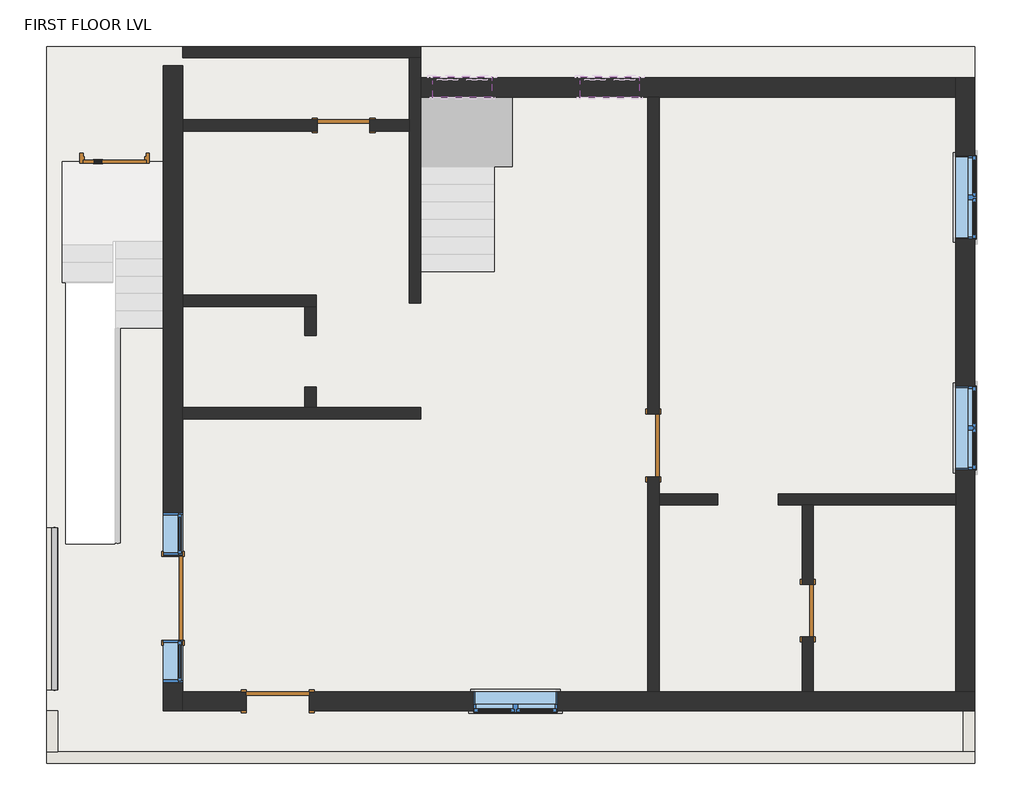
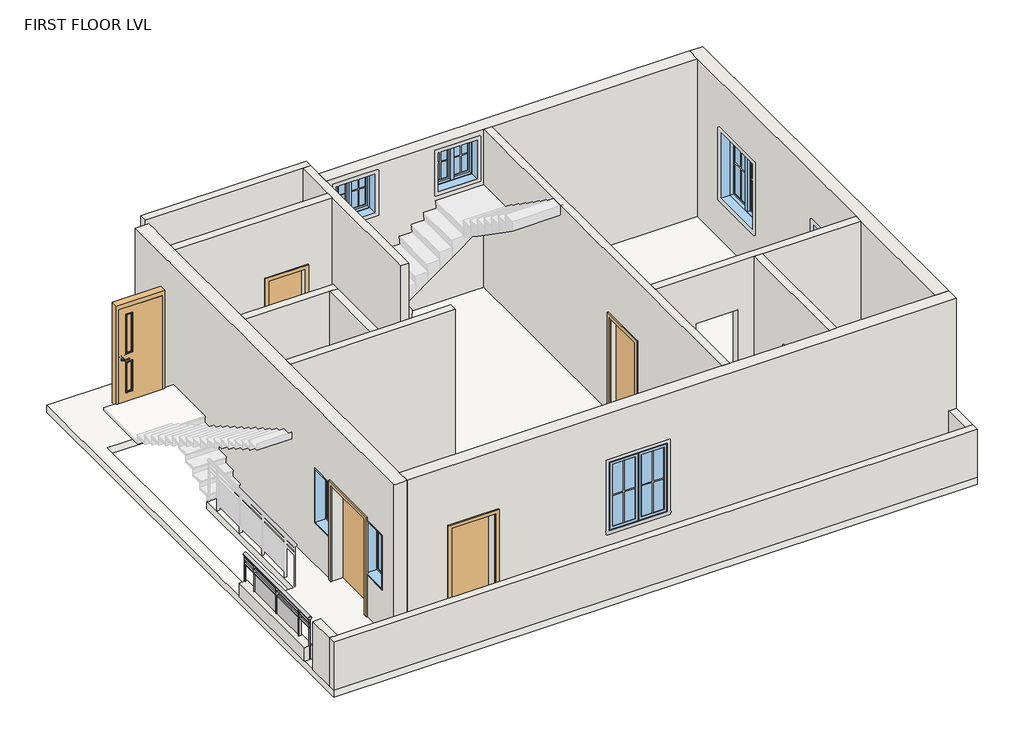
# One storey, part 1 of 2: 17 walls, 7 windows, 6 doors, 1 railing, 1 slab.
"""IFC4 building model written with IfcOpenShell, lengths in millimetres."""

from ifc_helpers import new_model, si_unit, point, frame, origin, place, context, project, spatial, polyline, ellipse_curve, trimmed, outline, extrude, faceted_brep, transform, mapped, element, save
from ifc_brep_helpers import plane_surface, extruded_surface, advanced_brep
from components import door_52fb15b9, door_3dc6c820, door_1da80235, door_d2d7de5b, door_21b9160b, window_dff46b58, window_6eb120d7, window_49c71971

model = new_model("IFC4")

# Units and contexts
model_context = context("Model", 3, world=origin())
ifc_project = project(units=[si_unit("LENGTHUNIT", "METRE", prefix="MILLI")], contexts=[model_context])

# Site, building, storey
site = spatial("IfcSite", under=ifc_project)
building = spatial("IfcBuilding", under=site)
storey = spatial("IfcBuildingStorey", under=building, Name="FIRST FLOOR LVL", Elevation=3505.2)

# Doors
placement = place(None, origin())
door_shape = door_52fb15b9(model_context)
element("IfcDoor", 1, ObjectType="Door-Passage-Single-Vision_Two_Lite : 36\" x 84\"", at=placement, inside=storey, context=model_context, shape_type="MappedRepresentation", body=[
    mapped(door_shape, transform((-6092.5155596, 7334.5576853, 4330.7), x_axis=(1.0, 0.0, 0.0), y_axis=(0.0, 1.0, 0.0), z_axis=(0.0, 0.0, 1.0))),
])
door_2_shape = door_3dc6c820(model_context)
element("IfcDoor", 2, ObjectType="Single-Flush : 30\" x 84\"", at=placement, inside=storey, context=model_context, shape_type="MappedRepresentation", body=[
    mapped(door_2_shape, transform((3997.6344404, 698.8076853, 3505.2), x_axis=(0.0, 1.0, 0.0), y_axis=(-1.0, 0.0, 0.0), z_axis=(0.0, 0.0, 1.0))),
])
element("IfcDoor", 3, ObjectType="Single-Flush : 30\" x 84\"", at=placement, inside=storey, context=model_context, shape_type="MappedRepresentation", body=[
    mapped(door_2_shape, transform((-2758.7655596, 7766.3576853, 3505.2), x_axis=(-1.0, 0.0, 0.0), y_axis=(0.0, -1.0, 0.0), z_axis=(0.0, 0.0, 1.0))),
])
door_3_shape = door_1da80235(model_context)
element("IfcDoor", 4, ObjectType="Single-Flush : 36\" x 84\"", at=placement, inside=storey, context=model_context, shape_type="MappedRepresentation", body=[
    mapped(door_3_shape, transform((-3717.6155596, -621.9923147, 3505.2), x_axis=(-1.0, 0.0, 0.0), y_axis=(0.0, -1.0, 0.0), z_axis=(0.0, 0.0, 1.0))),
])
door_4_shape = door_d2d7de5b(model_context)
element("IfcDoor", 5, ObjectType="Single-Flush : 36\" x 84\"", at=placement, inside=storey, context=model_context, shape_type="MappedRepresentation", body=[
    mapped(door_4_shape, transform((1749.7344404, 3105.4576853, 3505.2), x_axis=(0.0, -1.0, 0.0), y_axis=(1.0, 0.0, 0.0), z_axis=(0.0, 0.0, 1.0))),
])
door_5_shape = door_21b9160b(model_context)
element("IfcDoor", 6, ObjectType="Single-Flush : 48\" x 84\"", at=placement, inside=storey, context=model_context, shape_type="MappedRepresentation", body=[
    mapped(door_5_shape, transform((-5241.6155596, 876.6076853, 3505.2), x_axis=(0.0, -1.0, 0.0), y_axis=(1.0, 0.0, 0.0), z_axis=(0.0, 0.0, 1.0))),
])

# Railing
element("IfcRailing", 7, ObjectType="Glass Panel - Bottom Fill", at=placement, inside=storey, context=model_context, shape_type="SolidModel", body=[
    advanced_brep(
    [(-7006.9155596, -456.8923147, 4419.6), (-6930.7155596, -456.8923147, 4419.6), (-7006.9155596, 1905.3076853, 4419.6), (-6930.7155596, 1905.3076853, 4419.6)],
    [
        (0, 1, ellipse_curve(frame((-6968.8155596, -456.8923147, 4419.6), z_axis=(0.0, -1.0, 0.0), x_axis=(1.0, 0.0, 0.0)), 38.1, 28.575)),
        (1, 0, ellipse_curve(frame((-6968.8155596, -456.8923147, 4419.6), z_axis=(0.0, -1.0, 0.0), x_axis=(1.0, 0.0, 0.0)), 38.1, 28.575)),
        (2, 3, ellipse_curve(frame((-6968.8155596, 1905.3076853, 4419.6), z_axis=(0.0, 1.0, 0.0), x_axis=(1.0, 0.0, 0.0)), 38.1, 28.575)),
        (3, 2, ellipse_curve(frame((-6968.8155596, 1905.3076853, 4419.6), z_axis=(0.0, 1.0, 0.0), x_axis=(1.0, 0.0, 0.0)), 38.1, 28.575)),
        (0, 2),
        (3, 1),
    ],
    [
        plane_surface(frame((-6968.8155596, -456.8923147, 4419.6), z_axis=(0.0, -1.0, 0.0), x_axis=(0.0, 0.0, 1.0))),
        plane_surface(frame((-6968.8155596, 1905.3076853, 4419.6), z_axis=(0.0, 1.0, 0.0), x_axis=(0.0, 0.0, 1.0))),
        extruded_surface(trimmed(ellipse_curve(frame((-6968.8155596, 1905.3076853, 4419.6), z_axis=(0.0, -1.0, 0.0), x_axis=(1.0, 0.0, 0.0)), 38.1, 28.575), [point((-7006.9155596, 1905.3076853, 4419.6))], [point((-6930.7155596, 1905.3076853, 4419.6))], True, "CARTESIAN"), (0.0, -2362.2, 0.0), 2362.2),
        extruded_surface(trimmed(ellipse_curve(frame((-6968.8155596, 1905.3076853, 4419.6), z_axis=(0.0, -1.0, 0.0), x_axis=(1.0, 0.0, 0.0)), 38.1, 28.575), [point((-6930.7155596, 1905.3076853, 4419.6))], [point((-7006.9155596, 1905.3076853, 4419.6))], True, "CARTESIAN"), (0.0, -2362.2, 0.0), 2362.2),
    ],
    [
        (0, [[1, 2]]),
        (1, [[3, 4]]),
        (2, [[-1, 5, -4, 6]]),
        (3, [[-2, -6, -3, -5]]),
    ],
),
    extrude(outline(polyline([(-6956.1155596, -456.8923147), (-6981.5155596, -456.8923147), (-6981.5155596, 1905.3076853), (-6956.1155596, 1905.3076853), (-6956.1155596, -456.8923147)])), frame((0.0, 0.0, 4305.3), z_axis=(0.0, 0.0, 1.0), x_axis=(1.0, 0.0, 0.0)), (0.0, 0.0, 1.0), 25.4),
    extrude(outline(polyline([(-6956.1155596, -456.8923147), (-6981.5155596, -456.8923147), (-6981.5155596, 1905.3076853), (-6956.1155596, 1905.3076853), (-6956.1155596, -456.8923147)])), frame((0.0, 0.0, 4203.7), z_axis=(0.0, 0.0, 1.0), x_axis=(1.0, 0.0, 0.0)), (0.0, 0.0, 1.0), 25.4),
    extrude(outline(polyline([(-6943.4155596, 1530.6576853), (-6994.2155596, 1530.6576853), (-6994.2155596, 1543.3576853), (-6943.4155596, 1543.3576853), (-6943.4155596, 1530.6576853)])), frame((0.0, 0.0, 3505.2), z_axis=(0.0, 0.0, 1.0), x_axis=(1.0, 0.0, 0.0)), (0.0, 0.0, 1.0), 885.825),
    extrude(outline(polyline([(-6975.3507166, 724.2076853), (-6975.3507166, 1537.0076853), (-6969.0007166, 1537.0076853), (-6969.0007166, 724.2076853), (-6975.3507166, 724.2076853)])), frame((0.0, 0.0, 3606.8), z_axis=(0.0, 0.0, 1.0), x_axis=(1.0, 0.0, 0.0)), (0.0, 0.0, 1.0), 596.9),
    extrude(outline(polyline([(-6943.4155596, 717.8576853), (-6994.2155596, 717.8576853), (-6994.2155596, 730.5576853), (-6943.4155596, 730.5576853), (-6943.4155596, 717.8576853)])), frame((0.0, 0.0, 3505.2), z_axis=(0.0, 0.0, 1.0), x_axis=(1.0, 0.0, 0.0)), (0.0, 0.0, 1.0), 885.825),
    extrude(outline(polyline([(-6975.3507166, -88.5923147), (-6975.3507166, 724.2076853), (-6969.0007166, 724.2076853), (-6969.0007166, -88.5923147), (-6975.3507166, -88.5923147)])), frame((0.0, 0.0, 3606.8), z_axis=(0.0, 0.0, 1.0), x_axis=(1.0, 0.0, 0.0)), (0.0, 0.0, 1.0), 596.9),
    extrude(outline(polyline([(-6943.4155596, -94.9423147), (-6994.2155596, -94.9423147), (-6994.2155596, -82.2423147), (-6943.4155596, -82.2423147), (-6943.4155596, -94.9423147)])), frame((0.0, 0.0, 3505.2), z_axis=(0.0, 0.0, 1.0), x_axis=(1.0, 0.0, 0.0)), (0.0, 0.0, 1.0), 885.825),
    extrude(outline(polyline([(-6959.2905596, 1892.6076853), (-6978.3405596, 1892.6076853), (-6978.3405596, 1911.6576853), (-6959.2905596, 1911.6576853), (-6959.2905596, 1892.6076853)])), frame((0.0, 0.0, 3505.2), z_axis=(0.0, 0.0, 1.0), x_axis=(1.0, 0.0, 0.0)), (0.0, 0.0, 1.0), 885.825),
    extrude(outline(polyline([(-6959.2905596, -463.2423147), (-6978.3405596, -463.2423147), (-6978.3405596, -444.1923147), (-6959.2905596, -444.1923147), (-6959.2905596, -463.2423147)])), frame((0.0, 0.0, 3505.2), z_axis=(0.0, 0.0, 1.0), x_axis=(1.0, 0.0, 0.0)), (0.0, 0.0, 1.0), 885.825),
])

# Slab
element("IfcSlab", 8, ObjectType="Generic - 6\"", at=placement, inside=storey, context=model_context, shape_type="SweptSolid", body=[
    extrude(outline(polyline([(6429.6844404, 8915.7076853), (6429.6844404, -1523.6923147), (-7083.1155596, -1523.6923147), (-7083.1155596, 8915.7076853), (6429.6844404, 8915.7076853)]), holes=[polyline([(-6092.5155596, 1670.3576853), (-6092.5155596, 4813.6076853), (-5381.3155596, 4813.6076853), (-5381.3155596, 7188.5076853), (-6092.5155596, 7188.5076853), (-6803.7155596, 7188.5076853), (-6803.7155596, 1670.3576853), (-6092.5155596, 1670.3576853)])]), frame((0.0, 0.0, 3352.8), z_axis=(0.0, 0.0, 1.0), x_axis=(1.0, 0.0, 0.0)), (0.0, 0.0, 1.0), 152.4),
])

# Walls
element("IfcWall", 9, ObjectType="4", at=placement, inside=storey, context=model_context, shape_type="Brep", body=[
    faceted_brep([(-5101.9155596, 8750.6076853, 3505.2), (-1799.9155596, 8750.6076853, 3505.2), (-1634.8155596, 8750.6076853, 3505.2), (-1634.8155596, 8750.6076853, 7010.4), (-1799.9155596, 8750.6076853, 7010.4), (-5101.9155596, 8750.6076853, 7010.4), (-5101.9155596, 8915.7076853, 3505.2), (-5101.9155596, 8915.7076853, 7010.4), (-1634.8155596, 8915.7076853, 7010.4), (-1634.8155596, 8915.7076853, 3505.2)], [[[0, 1, 2, 3, 4, 5]], [[6, 7, 8, 9]], [[2, 1, 0, 6, 9]], [[5, 4, 3, 8, 7]], [[0, 5, 7, 6]], [[3, 2, 9, 8]]]),
])
element("IfcWall", 10, ObjectType="4", at=placement, inside=storey, context=model_context, shape_type="Brep", body=[
    faceted_brep([(-1799.9155596, 8750.6076853, 3505.2), (-1799.9155596, 8458.5076853, 3505.2), (-1799.9155596, 8229.9076853, 3505.2), (-1799.9155596, 7848.9076853, 3505.2), (-1799.9155596, 7683.8076853, 3505.2), (-1799.9155596, 5410.5076853, 3505.2), (-1799.9155596, 5181.9076853, 3505.2), (-1799.9155596, 5181.9076853, 7010.4), (-1799.9155596, 7683.8076853, 7010.4), (-1799.9155596, 7848.9076853, 7010.4), (-1799.9155596, 8229.9076853, 7010.4), (-1799.9155596, 8458.5076853, 7010.4), (-1799.9155596, 8750.6076853, 7010.4), (-1634.8155596, 8750.6076853, 3505.2), (-1634.8155596, 8750.6076853, 7010.4), (-1634.8155596, 8458.5076853, 7010.4), (-1634.8155596, 8179.1076853, 7010.4), (-1634.8155596, 5181.9076853, 7010.4), (-1634.8155596, 5181.9076853, 3505.2), (-1634.8155596, 5410.5076853, 3505.2), (-1634.8155596, 8179.1076853, 3505.2), (-1634.8155596, 8229.9076853, 3505.2), (-1634.8155596, 8458.5076853, 3505.2)], [[[0, 1, 2, 3, 4, 5, 6, 7, 8, 9, 10, 11, 12]], [[13, 14, 15, 16, 17, 18, 19, 20, 21, 22]], [[6, 5, 4, 3, 2, 1, 0, 13, 22, 21, 20, 19, 18]], [[7, 6, 18, 17]], [[12, 11, 10, 9, 8, 7, 17, 16, 15, 14]], [[0, 12, 14, 13]]]),
])
element("IfcWall", 11, ObjectType="4", at=placement, inside=storey, context=model_context, shape_type="SweptSolid", body=[
    extrude(outline(polyline([(3505.2, -5101.9155596), (3505.2, -3139.7655596), (5638.8, -3139.7655596), (5638.8, -2377.7655596), (3505.2, -2377.7655596), (3505.2, -1799.9155596), (7010.4, -1799.9155596), (7010.4, -5101.9155596), (3505.2, -5101.9155596)])), frame((0.0, 7683.8076853, 0.0), z_axis=(0.0, 1.0, 0.0), x_axis=(0.0, 0.0, 1.0)), (0.0, 0.0, 1.0), 165.1),
])
element("IfcWall", 12, ObjectType="4", at=placement, inside=storey, context=model_context, shape_type="Brep", body=[
    faceted_brep([(-5101.9155596, 5131.1076853, 3505.2), (-3323.9155596, 5131.1076853, 3505.2), (-3158.8155596, 5131.1076853, 3505.2), (-3158.8155596, 5131.1076853, 7010.4), (-3323.9155596, 5131.1076853, 7010.4), (-5101.9155596, 5131.1076853, 7010.4), (-5101.9155596, 5296.2076853, 3505.2), (-5101.9155596, 5296.2076853, 7010.4), (-3158.8155596, 5296.2076853, 7010.4), (-3158.8155596, 5296.2076853, 3505.2)], [[[0, 1, 2, 3, 4, 5]], [[6, 7, 8, 9]], [[2, 1, 0, 6, 9]], [[5, 4, 3, 8, 7]], [[0, 5, 7, 6]], [[3, 2, 9, 8]]]),
])
element("IfcWall", 13, ObjectType="4", at=placement, inside=storey, context=model_context, shape_type="SweptSolid", body=[
    extrude(outline(polyline([(3657.9076853, 3505.2), (3657.9076853, 7010.4), (5131.1076853, 7010.4), (5131.1076853, 3505.2), (4705.6576853, 3505.2), (4705.6576853, 5943.6), (3956.3576853, 5943.6), (3956.3576853, 3505.2), (3657.9076853, 3505.2)])), frame((-3323.9155596, 0.0, 0.0), z_axis=(1.0, 0.0, 0.0), x_axis=(0.0, 1.0, 0.0)), (0.0, 0.0, 1.0), 165.1),
])
element("IfcWall", 14, ObjectType="4", at=placement, inside=storey, context=model_context, shape_type="Brep", body=[
    faceted_brep([(1667.1844404, 2648.2576853, 5638.8), (1667.1844404, 2648.2576853, 3505.2), (1667.1844404, -482.2923147, 3505.2), (1667.1844404, -482.2923147, 7010.4), (1667.1844404, 8179.1076853, 7010.4), (1667.1844404, 8179.1076853, 3505.2), (1667.1844404, 3562.6576853, 3505.2), (1667.1844404, 3562.6576853, 5638.8), (1832.2844404, -482.2923147, 3505.2), (1832.2844404, 2235.5076853, 3505.2), (1832.2844404, 2400.6076853, 3505.2), (1832.2844404, 2514.9076853, 3505.2), (1832.2844404, 2648.2576853, 3505.2), (1832.2844404, 2648.2576853, 5638.8), (1832.2844404, 3562.6576853, 5638.8), (1832.2844404, 3562.6576853, 3505.2), (1832.2844404, 5181.9076853, 3505.2), (1832.2844404, 5410.5076853, 3505.2), (1832.2844404, 8179.1076853, 3505.2), (1832.2844404, 8179.1076853, 7010.4), (1832.2844404, 2400.6076853, 7010.4), (1832.2844404, 2235.5076853, 7010.4), (1832.2844404, -482.2923147, 7010.4)], [[[0, 1, 2, 3, 4, 5, 6, 7]], [[8, 9, 10, 11, 12, 13, 14, 15, 16, 17, 18, 19, 20, 21, 22]], [[6, 5, 18, 17, 16, 15]], [[2, 1, 12, 11, 10, 9, 8]], [[4, 3, 22, 21, 20, 19]], [[3, 2, 8, 22]], [[5, 4, 19, 18]], [[13, 12, 1, 0]], [[14, 13, 0, 7]], [[15, 14, 7, 6]]]),
])
element("IfcWall", 15, ObjectType="4", at=placement, inside=storey, context=model_context, shape_type="SweptSolid", body=[
    extrude(outline(polyline([(2235.5076853, 3505.2), (1079.8076853, 3505.2), (1079.8076853, 5638.8), (317.8076853, 5638.8), (317.8076853, 3505.2), (-482.2923147, 3505.2), (-482.2923147, 7010.4), (2235.5076853, 7010.4), (2235.5076853, 3505.2)])), frame((3915.0844404, 0.0, 0.0), z_axis=(1.0, 0.0, 0.0), x_axis=(0.0, 1.0, 0.0)), (0.0, 0.0, 1.0), 165.1),
])
element("IfcWall", 16, ObjectType="4", at=placement, inside=storey, context=model_context, shape_type="Brep", body=[
    faceted_brep([(6150.2844404, 2235.5076853, 3505.2), (6150.2844404, 2235.5076853, 7010.4), (4080.1844404, 2235.5076853, 7010.4), (3915.0844404, 2235.5076853, 7010.4), (1832.2844404, 2235.5076853, 7010.4), (1832.2844404, 2235.5076853, 3505.2), (2687.0502939, 2235.5076853, 3505.2), (2687.0502939, 2235.5076853, 5943.6), (3567.6284806, 2235.5076853, 5943.6), (3567.6284806, 2235.5076853, 3505.2), (3915.0844404, 2235.5076853, 3505.2), (4080.1844404, 2235.5076853, 3505.2), (6150.2844404, 2400.6076853, 7010.4), (6150.2844404, 2400.6076853, 3505.2), (5611.8165832, 2400.6076853, 3505.2), (5307.0165832, 2400.6076853, 3505.2), (3567.6284806, 2400.6076853, 3505.2), (3567.6284806, 2400.6076853, 5943.6), (2687.0502939, 2400.6076853, 5943.6), (2687.0502939, 2400.6076853, 3505.2), (2022.7844404, 2400.6076853, 3505.2), (1832.2844404, 2400.6076853, 3505.2), (1832.2844404, 2400.6076853, 7010.4)], [[[0, 1, 2, 3, 4, 5, 6, 7, 8, 9, 10, 11]], [[12, 13, 14, 15, 16, 17, 18, 19, 20, 21, 22]], [[5, 21, 20, 19, 6]], [[13, 0, 11, 10, 9, 16, 15, 14]], [[4, 3, 2, 1, 12, 22]], [[1, 0, 13, 12]], [[5, 4, 22, 21]], [[7, 18, 17, 8]], [[18, 7, 6, 19]], [[8, 17, 16, 9]]]),
])
element("IfcWall", 17, ObjectType="4", at=placement, inside=storey, context=model_context, shape_type="Brep", body=[
    faceted_brep([(-5101.9155596, 3492.8076853, 3505.2), (-1634.8155596, 3492.8076853, 3505.2), (-1634.8155596, 3492.8076853, 7010.4), (-5101.9155596, 3492.8076853, 7010.4), (-5101.9155596, 3657.9076853, 3505.2), (-5101.9155596, 3657.9076853, 7010.4), (-3323.9155596, 3657.9076853, 7010.4), (-3158.8155596, 3657.9076853, 7010.4), (-1634.8155596, 3657.9076853, 7010.4), (-1634.8155596, 3657.9076853, 3505.2), (-3158.8155596, 3657.9076853, 3505.2), (-3323.9155596, 3657.9076853, 3505.2)], [[[0, 1, 2, 3]], [[4, 5, 6, 7, 8, 9, 10, 11]], [[1, 0, 4, 11, 10, 9]], [[2, 1, 9, 8]], [[3, 2, 8, 7, 6, 5]], [[0, 3, 5, 4]]]),
])
element("IfcWall", 18, ObjectType="4", at=placement, inside=storey, context=model_context, shape_type="Brep", body=[
    faceted_brep([(6429.6844404, -1358.5923147, 3505.2), (6264.5844404, -1358.5923147, 3505.2), (-6918.0155596, -1358.5923147, 3505.2), (-7083.1155596, -1358.5923147, 3505.2), (-7083.1155596, -1358.5923147, 4572.0), (-6918.0155596, -1358.5923147, 4572.0), (6264.5844404, -1358.5923147, 4572.0), (6429.6844404, -1358.5923147, 4572.0), (6429.6844404, -1523.6923147, 3505.2), (6429.6844404, -1523.6923147, 4572.0), (-7083.1155596, -1523.6923147, 4572.0), (-7083.1155596, -1523.6923147, 3505.2)], [[[0, 1, 2, 3, 4, 5, 6, 7]], [[8, 9, 10, 11]], [[3, 2, 1, 0, 8, 11]], [[7, 6, 5, 4, 10, 9]], [[4, 3, 11, 10]], [[0, 7, 9, 8]]]),
])
element("IfcWall", 19, ObjectType="4", at=placement, inside=storey, context=model_context, shape_type="SweptSolid", body=[
    extrude(outline(polyline([(-6918.0155596, -761.6923147), (-6918.0155596, -1358.5923147), (-7083.1155596, -1358.5923147), (-7083.1155596, -761.6923147), (-6918.0155596, -761.6923147)])), frame((0.0, 0.0, 3505.2), z_axis=(0.0, 0.0, 1.0), x_axis=(1.0, 0.0, 0.0)), (0.0, 0.0, 1.0), 1066.8),
])
element("IfcWall", 20, ObjectType="4", at=placement, inside=storey, context=model_context, shape_type="SweptSolid", body=[
    extrude(outline(polyline([(-6918.0155596, 1905.3076853), (-6918.0155596, -456.8923147), (-7083.1155596, -456.8923147), (-7083.1155596, 1905.3076853), (-6918.0155596, 1905.3076853)])), frame((0.0, 0.0, 3505.2), z_axis=(0.0, 0.0, 1.0), x_axis=(1.0, 0.0, 0.0)), (0.0, 0.0, 1.0), 304.8),
])
element("IfcWall", 21, ObjectType="4", at=placement, inside=storey, context=model_context, shape_type="SweptSolid", body=[
    extrude(outline(polyline([(6429.6844404, -761.6923147), (6429.6844404, -1358.5923147), (6264.5844404, -1358.5923147), (6264.5844404, -761.6923147), (6429.6844404, -761.6923147)])), frame((0.0, 0.0, 3505.2), z_axis=(0.0, 0.0, 1.0), x_axis=(1.0, 0.0, 0.0)), (0.0, 0.0, 1.0), 1066.8),
])
element("IfcWall", 22, ObjectType="9", at=placement, inside=storey, context=model_context, shape_type="Brep", body=[
    faceted_brep([(-5381.3155596, -761.6923147, 7010.4), (-5381.3155596, 8636.3076853, 7010.4), (-5381.3155596, 8636.3076853, 3505.2), (-5381.3155596, 7467.9076853, 3505.2), (-5381.3155596, 7188.5076853, 3505.2), (-5381.3155596, 1486.2076853, 3505.2), (-5381.3155596, 1486.2076853, 5638.8), (-5381.3155596, -342.5923147, 5638.8), (-5381.3155596, -342.5923147, 4419.6), (-5381.3155596, 267.0076853, 4419.6), (-5381.3155596, 267.0076853, 3505.2), (-5381.3155596, -761.6923147, 3505.2), (-5381.3155596, 1511.6076853, 5638.8), (-5381.3155596, 1511.6076853, 4419.6), (-5381.3155596, 2121.2076853, 4419.6), (-5381.3155596, 2121.2076853, 5638.8), (-5101.9155596, 8636.3076853, 7010.4), (-5101.9155596, 8458.5076853, 7010.4), (-5101.9155596, 8229.9076853, 7010.4), (-5101.9155596, 7848.9076853, 7010.4), (-5101.9155596, 7683.8076853, 7010.4), (-5101.9155596, 5296.2076853, 7010.4), (-5101.9155596, 5131.1076853, 7010.4), (-5101.9155596, 3657.9076853, 7010.4), (-5101.9155596, 3492.8076853, 7010.4), (-5101.9155596, -456.8923147, 7010.4), (-5101.9155596, -482.2923147, 7010.4), (-5101.9155596, -761.6923147, 7010.4), (-5101.9155596, -761.6923147, 3505.2), (-5101.9155596, -482.2923147, 3505.2), (-5101.9155596, -456.8923147, 3505.2), (-5101.9155596, 267.0076853, 3505.2), (-5101.9155596, 267.0076853, 4419.6), (-5101.9155596, -342.5923147, 4419.6), (-5101.9155596, -342.5923147, 5638.8), (-5101.9155596, 1486.2076853, 5638.8), (-5101.9155596, 1486.2076853, 3505.2), (-5101.9155596, 3492.8076853, 3505.2), (-5101.9155596, 3657.9076853, 3505.2), (-5101.9155596, 5131.1076853, 3505.2), (-5101.9155596, 5181.9076853, 3505.2), (-5101.9155596, 5296.2076853, 3505.2), (-5101.9155596, 5486.7076853, 3505.2), (-5101.9155596, 7683.8076853, 3505.2), (-5101.9155596, 7848.9076853, 3505.2), (-5101.9155596, 8229.9076853, 3505.2), (-5101.9155596, 8458.5076853, 3505.2), (-5101.9155596, 8636.3076853, 3505.2), (-5101.9155596, 1511.6076853, 5638.8), (-5101.9155596, 2121.2076853, 5638.8), (-5101.9155596, 2121.2076853, 4419.6), (-5101.9155596, 1511.6076853, 4419.6), (-5241.6155596, 8636.3076853, 3505.2), (-5330.5155596, -761.6923147, 3505.2), (-5330.5155596, -761.6923147, 7010.4)], [[[0, 1, 2, 3, 4, 5, 6, 7, 8, 9, 10, 11], [12, 13, 14, 15]], [[16, 17, 18, 19, 20, 21, 22, 23, 24, 25, 26, 27, 28, 29, 30, 31, 32, 33, 34, 35, 36, 37, 38, 39, 40, 41, 42, 43, 44, 45, 46, 47], [48, 49, 50, 51]], [[2, 52, 47, 46, 45, 44, 43, 42, 41, 40, 39, 38, 37, 36, 5, 4, 3]], [[28, 53, 11, 10, 31, 30, 29]], [[1, 0, 54, 27, 26, 25, 24, 23, 22, 21, 20, 19, 18, 17, 16]], [[2, 1, 16, 47, 52]], [[0, 11, 53, 28, 27, 54]], [[31, 10, 9, 32]], [[34, 7, 6, 35]], [[36, 35, 6, 5]], [[13, 12, 48, 51]], [[14, 13, 51, 50]], [[15, 14, 50, 49]], [[12, 15, 49, 48]], [[7, 34, 33, 8]], [[8, 33, 32, 9]]]),
])
element("IfcWall", 23, ObjectType="9", at=placement, inside=storey, context=model_context, shape_type="Brep", body=[
    faceted_brep([(-5101.9155596, -761.6923147, 3505.2), (-4174.8155596, -761.6923147, 3505.2), (-4174.8155596, -761.6923147, 5638.8), (-3260.4155596, -761.6923147, 5638.8), (-3260.4155596, -761.6923147, 3505.2), (-1939.6155596, -761.6923147, 3505.2), (-1634.8155596, -761.6923147, 3505.2), (1805.5088354, -761.6923147, 3505.2), (2110.3088354, -761.6923147, 3505.2), (5406.3209761, -761.6923147, 3505.2), (5711.1209761, -761.6923147, 3505.2), (6264.5844404, -761.6923147, 3505.2), (6429.6844404, -761.6923147, 3505.2), (6429.6844404, -761.6923147, 4572.0), (6429.6844404, -761.6923147, 7010.4), (-5101.9155596, -761.6923147, 7010.4), (-866.4655596, -761.6923147, 5943.6), (352.7344404, -761.6923147, 5943.6), (352.7344404, -761.6923147, 4419.6), (-866.4655596, -761.6923147, 4419.6), (-4174.8155596, -482.2923147, 5638.8), (-4174.8155596, -482.2923147, 3505.2), (-5101.9155596, -482.2923147, 3505.2), (-5101.9155596, -482.2923147, 7010.4), (1667.1844404, -482.2923147, 7010.4), (1832.2844404, -482.2923147, 7010.4), (3915.0844404, -482.2923147, 7010.4), (4080.1844404, -482.2923147, 7010.4), (6150.2844404, -482.2923147, 7010.4), (6429.6844404, -482.2923147, 7010.4), (6429.6844404, -482.2923147, 3505.2), (6150.2844404, -482.2923147, 3505.2), (4080.1844404, -482.2923147, 3505.2), (3915.0844404, -482.2923147, 3505.2), (1832.2844404, -482.2923147, 3505.2), (1667.1844404, -482.2923147, 3505.2), (-3260.4155596, -482.2923147, 3505.2), (-3260.4155596, -482.2923147, 5638.8), (-866.4655596, -482.2923147, 5943.6), (-866.4655596, -482.2923147, 4419.6), (352.7344404, -482.2923147, 4419.6), (352.7344404, -482.2923147, 5943.6)], [[[0, 1, 2, 3, 4, 5, 6, 7, 8, 9, 10, 11, 12, 13, 14, 15], [16, 17, 18, 19]], [[20, 21, 22, 23, 24, 25, 26, 27, 28, 29, 30, 31, 32, 33, 34, 35, 36, 37], [38, 39, 40, 41]], [[22, 21, 1, 0]], [[36, 35, 34, 33, 32, 31, 30, 12, 11, 10, 9, 8, 7, 6, 5, 4]], [[15, 14, 29, 28, 27, 26, 25, 24, 23]], [[0, 15, 23, 22]], [[2, 1, 21, 20]], [[3, 2, 20, 37]], [[4, 3, 37, 36]], [[39, 38, 16, 19]], [[40, 39, 19, 18]], [[41, 40, 18, 17]], [[38, 41, 17, 16]], [[12, 30, 29, 14, 13]]]),
])
element("IfcWall", 24, ObjectType="9", at=placement, inside=storey, context=model_context, shape_type="Brep", body=[
    faceted_brep([(6429.6844404, -482.2923147, 7010.4), (6429.6844404, -482.2923147, 3505.2), (6429.6844404, 8458.5076853, 3505.2), (6429.6844404, 8458.5076853, 7010.4), (6429.6844404, 2749.8576853, 5943.6), (6429.6844404, 3969.0576853, 5943.6), (6429.6844404, 3969.0576853, 4419.6), (6429.6844404, 2749.8576853, 4419.6), (6429.6844404, 6109.0076853, 5943.6), (6429.6844404, 7328.2076853, 5943.6), (6429.6844404, 7328.2076853, 4419.6), (6429.6844404, 6109.0076853, 4419.6), (6150.2844404, -482.2923147, 3505.2), (6150.2844404, -482.2923147, 7010.4), (6150.2844404, 2235.5076853, 7010.4), (6150.2844404, 2400.6076853, 7010.4), (6150.2844404, 8179.1076853, 7010.4), (6150.2844404, 8458.5076853, 7010.4), (6150.2844404, 8458.5076853, 3505.2), (6150.2844404, 8179.1076853, 3505.2), (6150.2844404, 2400.6076853, 3505.2), (6150.2844404, 2235.5076853, 3505.2), (6150.2844404, 2749.8576853, 5943.6), (6150.2844404, 2749.8576853, 4419.6), (6150.2844404, 3969.0576853, 4419.6), (6150.2844404, 3969.0576853, 5943.6), (6150.2844404, 6109.0076853, 5943.6), (6150.2844404, 6109.0076853, 4419.6), (6150.2844404, 7328.2076853, 4419.6), (6150.2844404, 7328.2076853, 5943.6)], [[[0, 1, 2, 3], [4, 5, 6, 7], [8, 9, 10, 11]], [[12, 13, 14, 15, 16, 17, 18, 19, 20, 21], [22, 23, 24, 25], [26, 27, 28, 29]], [[2, 1, 12, 21, 20, 19, 18]], [[0, 3, 17, 16, 15, 14, 13]], [[3, 2, 18, 17]], [[23, 22, 4, 7]], [[24, 23, 7, 6]], [[25, 24, 6, 5]], [[22, 25, 5, 4]], [[27, 26, 8, 11]], [[28, 27, 11, 10]], [[29, 28, 10, 9]], [[26, 29, 9, 8]], [[0, 13, 12, 1]]]),
])
element("IfcWall", 25, ObjectType="9", at=placement, inside=storey, context=model_context, shape_type="Brep", body=[
    faceted_brep([(6150.2844404, 8458.5076853, 3505.2), (5611.8165832, 8458.5076853, 3505.2), (5307.0165832, 8458.5076853, 3505.2), (2022.7844404, 8458.5076853, 3505.2), (1717.9844404, 8458.5076853, 3505.2), (-1634.8155596, 8458.5076853, 3505.2), (-1634.8155596, 8458.5076853, 7010.4), (6150.2844404, 8458.5076853, 7010.4), (-599.7655596, 8458.5076853, 6858.0), (-1463.3655596, 8458.5076853, 6858.0), (-1463.3655596, 8458.5076853, 5943.6), (-599.7655596, 8458.5076853, 5943.6), (1546.5344404, 8458.5076853, 6858.0), (682.9344404, 8458.5076853, 6858.0), (682.9344404, 8458.5076853, 5943.6), (1546.5344404, 8458.5076853, 5943.6), (6150.2844404, 8179.1076853, 3505.2), (6150.2844404, 8179.1076853, 7010.4), (1832.2844404, 8179.1076853, 7010.4), (1667.1844404, 8179.1076853, 7010.4), (-1634.8155596, 8179.1076853, 7010.4), (-1634.8155596, 8179.1076853, 3505.2), (1667.1844404, 8179.1076853, 3505.2), (1832.2844404, 8179.1076853, 3505.2), (-599.7655596, 8179.1076853, 6858.0), (-599.7655596, 8179.1076853, 5943.6), (-1463.3655596, 8179.1076853, 5943.6), (-1463.3655596, 8179.1076853, 6858.0), (1546.5344404, 8179.1076853, 6858.0), (1546.5344404, 8179.1076853, 5943.6), (682.9344404, 8179.1076853, 5943.6), (682.9344404, 8179.1076853, 6858.0)], [[[0, 1, 2, 3, 4, 5, 6, 7], [8, 9, 10, 11], [12, 13, 14, 15]], [[16, 17, 18, 19, 20, 21, 22, 23], [24, 25, 26, 27], [28, 29, 30, 31]], [[5, 4, 3, 2, 1, 0, 16, 23, 22, 21]], [[7, 6, 20, 19, 18, 17]], [[0, 7, 17, 16]], [[6, 5, 21, 20]], [[25, 24, 8, 11]], [[26, 25, 11, 10]], [[27, 26, 10, 9]], [[24, 27, 9, 8]], [[29, 28, 12, 15]], [[30, 29, 15, 14]], [[31, 30, 14, 13]], [[28, 31, 13, 12]]]),
])

# Windows
window_shape = window_dff46b58(model_context)
element("IfcWindow", 26, ObjectType="Fixed : 24\" x 48\"", at=placement, inside=storey, context=model_context, shape_type="MappedRepresentation", body=[
    mapped(window_shape, transform((-5241.6155596, 1778.3076853, 3505.2), x_axis=(0.0, -1.0, 0.0), y_axis=(1.0, 0.0, 0.0), z_axis=(0.0, 0.0, 1.0))),
])
element("IfcWindow", 27, ObjectType="Fixed : 24\" x 48\"", at=placement, inside=storey, context=model_context, shape_type="MappedRepresentation", body=[
    mapped(window_shape, transform((-5241.6155596, -75.8923147, 3505.2), x_axis=(0.0, -1.0, 0.0), y_axis=(1.0, 0.0, 0.0), z_axis=(0.0, 0.0, 1.0))),
])
window_2_shape = window_6eb120d7(model_context)
element("IfcWindow", 28, ObjectType="Window-Casement-Double : 34\" x 36\"", at=placement, inside=storey, context=model_context, shape_type="MappedRepresentation", body=[
    mapped(window_2_shape, transform((-1031.5655596, 8318.8076853, 5029.2), x_axis=(1.0, 0.0, 0.0), y_axis=(0.0, 1.0, 0.0), z_axis=(0.0, 0.0, 1.0))),
])
element("IfcWindow", 29, ObjectType="Window-Casement-Double : 34\" x 36\"", at=placement, inside=storey, context=model_context, shape_type="MappedRepresentation", body=[
    mapped(window_2_shape, transform((1114.7344404, 8318.8076853, 5029.2), x_axis=(1.0, 0.0, 0.0), y_axis=(0.0, 1.0, 0.0), z_axis=(0.0, 0.0, 1.0))),
])
window_3_shape = window_49c71971(model_context)
element("IfcWindow", 30, ObjectType="Window-Casement-Double : 48\" x 60\"", at=placement, inside=storey, context=model_context, shape_type="MappedRepresentation", body=[
    mapped(window_3_shape, transform((-256.8655596, -621.9923147, 3505.2), x_axis=(-1.0, 0.0, 0.0), y_axis=(0.0, -1.0, 0.0), z_axis=(0.0, 0.0, 1.0))),
])
element("IfcWindow", 31, ObjectType="Window-Casement-Double : 48\" x 60\"", at=placement, inside=storey, context=model_context, shape_type="MappedRepresentation", body=[
    mapped(window_3_shape, transform((6289.9844404, 3359.4576853, 3505.2), x_axis=(0.0, -1.0, 0.0), y_axis=(1.0, 0.0, 0.0), z_axis=(0.0, 0.0, 1.0))),
])
element("IfcWindow", 32, ObjectType="Window-Casement-Double : 48\" x 60\"", at=placement, inside=storey, context=model_context, shape_type="MappedRepresentation", body=[
    mapped(window_3_shape, transform((6289.9844404, 6718.6076853, 3505.2), x_axis=(0.0, -1.0, 0.0), y_axis=(1.0, 0.0, 0.0), z_axis=(0.0, 0.0, 1.0))),
])

save(model, "model.ifc")

# Revit data of these elements
# Type "Door-Passage-Single-Vision_Two_Lite : 36\" x 84\""
#   Type Mark = "9"
#   Assembly Code = "B2030100"
#   Analytic Construction = "Wooden"
#   Thickness = 0' - 1 3/4"
#   Thermal Resistance (R) = 2.5876 (h·ft²·°F)/BTU
#   Swing Angle [instance default] = 90.00°
#   Strike Height = 3' - 4"
#   Rough Width [instance default] = 3' - 4"
#   Rough Height [instance default] = 7' - 4"
#   MF Opening Height [instance default] = 0' - 4"
#   MF Opening Width [instance default] = 0' - 4"
#   Heat Transfer Coefficient (U) = 0.3865 BTU/(h·ft²·°F)
#   Inset Calculate [instance default] = 0' - 4"
#   Masonry Inset [instance default] = 0' - 1"
#   Height = 7' - 0"
#   Width = 3' - 0"
#   Masonry Frame Depth = 0' - 5 3/4"
#   Masonry Frame [instance default] = yes
#   Function = 1
#   Dry Wall Frame [instance default] = no
#   Panel Material = Wood - Birch
#   Glazing = Glass
#   Glass Stop Material = Metal - Paint Finish - Grey
#   Frame Material = Metal - Paint Finish - Grey
#   Door Handle Material = Aluminum
#   Visual Light Transmittance = 0
#   Solar Heat Gain Coefficient = 0
#   Wall Closure = (empty or 0)
# Type "Single-Flush : 30\" x 84\""
#   Type Mark = "4"
#   Construction Type Id = "MDOOR"
#   Assembly Code = "C1020"
#   Analytic Construction = "Metal"
#   Thickness = 0' - 2"
#   Heat Transfer Coefficient (U) = 0.651978 BTU/(h·ft²·°F)
#   Height = 7' - 0"
#   Trim Projection Ext = 0' - 1"
#   Trim Projection Int = 0' - 1"
#   Trim Width = 0' - 3"
#   Width = 2' - 6"
#   Define Thermal Properties by = 1
#   Define Thermal Properties by = 1
#   Door Material = Door - Panel
#   Frame Material = Door - Frame
#   Visual Light Transmittance = 0
#   Solar Heat Gain Coefficient = 0
#   Function = (empty or 0)
#   Wall Closure = (empty or 0)
# Type "Single-Flush : 36\" x 84\""
#   Type Mark = "1"
#   Construction Type Id = "MDOOR"
#   Assembly Code = "C1020"
#   Analytic Construction = "Metal"
#   Thickness = 0' - 2"
#   Heat Transfer Coefficient (U) = 0.651978 BTU/(h·ft²·°F)
#   Height = 7' - 0"
#   Trim Projection Ext = 0' - 1"
#   Trim Projection Int = 0' - 1"
#   Trim Width = 0' - 3"
#   Width = 3' - 0"
#   Define Thermal Properties by = 1
#   Define Thermal Properties by = 1
#   Door Material = Door - Panel
#   Frame Material = Door - Frame
#   Visual Light Transmittance = 0
#   Solar Heat Gain Coefficient = 0
#   Function = (empty or 0)
#   Wall Closure = (empty or 0)
# Type "Single-Flush : 48\" x 84\""
#   Type Mark = "8"
#   Construction Type Id = "MDOOR"
#   Assembly Code = "C1020"
#   Analytic Construction = "Metal"
#   Thickness = 0' - 2"
#   Heat Transfer Coefficient (U) = 0.651978 BTU/(h·ft²·°F)
#   Height = 7' - 0"
#   Trim Projection Ext = 0' - 1"
#   Trim Projection Int = 0' - 1"
#   Trim Width = 0' - 3"
#   Width = 4' - 0"
#   Define Thermal Properties by = 1
#   Door Material = Door - Panel
#   Frame Material = Door - Frame
#   Visual Light Transmittance = 0
#   Solar Heat Gain Coefficient = 0
#   Function = (empty or 0)
#   Wall Closure = (empty or 0)
# Type "Glass Panel - Bottom Fill"
#   Assembly Code = "C2010400"
#   built-in parameter 1008612 = 0.0416667 (stored number, unit not read)
#   built-in parameter 1008611 = 0.0416667 (stored number, unit not read)
#   built-in parameter 1008609 = 0.333333 (stored number, unit not read)
#   built-in parameter 1008604 = 0.166667 (stored number, unit not read)
#   built-in parameter 1008603 = 0.166667 (stored number, unit not read)
#   Railing Height = 3' - 0"
#   built-in parameter 1008630 = 2
#   built-in parameter 1008610 = 2
#   built-in parameter 1008618 = Baluster - Square : 3/4"
# Type "Generic - 6\""
#   Assembly Code = "B1010"
#   Function = 0
#   Layers, outside or top first: 0' - 6" no material (function 1)
# Type "4"
#   Assembly Code = "B2010"
#   Layers, outside or top first: 0' - 1" "Gypsum Wall Board" (function 1); 0' - 4 1/2" no material (function 1); 0' - 1" "Gypsum Wall Board" (function 1)
# Type "9"
#   Assembly Code = "B2010"
#   Layers, outside or top first: 0' - 1" "Gypsum Wall Board" (function 1); 0' - 9" no material (function 1); 0' - 1" "Gypsum Wall Board" (function 1)
# Type "Fixed : 24\" x 48\""
#   Type Mark = "2"
#   Construction Type Id = "GSP4R"
#   Assembly Code = "B2020100"
#   Analytic Construction = "1/8 in Pilkington single glazing"
#   Visual Light Transmittance = 0.9
#   Solar Heat Gain Coefficient = 0.78
#   Heat Transfer Coefficient (U) = 0.6496 BTU/(h·ft²·°F)
#   Height = 4' - 0"
#   Default Sill Height = 3' - 0"
#   Width = 2' - 0"
#   Window Inset = 0' - 0 3/4"
#   Define Thermal Properties by = 1
#   Define Thermal Properties by = 1
#   Glass Pane Material = Glass
#   Sash Material = Sash
#   Wall Closure = (empty or 0)
# Type "Window-Casement-Double : 34\" x 36\""
#   Type Mark = "14"
#   Fire Rating = "0.5h"
#   Assembly Code = "B2020100"
#   Analytic Construction = "Double glazing - domestic"
#   Frame Extension [instance default] = 0' - 0 1/4"
#   Window Inset [instance default] = 0' - 0"
#   Wall Thickness [instance default] = 0' - 6"
#   Interior Wall Closure [instance default] = 0' - 2 1/4"
#   Half Width = 1' - 5"
#   Visual Light Transmittance = 0.81
#   Thermal Resistance (R) = 1.8146 (h·ft²·°F)/BTU
#   Solar Heat Gain Coefficient = 0.76
#   Rough Width = 2' - 10 1/2"
#   Rough Height = 3' - 0 1/2"
#   Height = 3' - 0"
#   Heat Transfer Coefficient (U) = 0.5511 BTU/(h·ft²·°F)
#   Exterior Wall Closure [instance default] = 0' - 1 1/4"
#   Extension Jamb [instance default] = 0' - 2 1/4"
#   Default Sill Height = 3' - 0"
#   Width = 2' - 10"
#   Define Thermal Properties by = 0
#   Muntin Visibility = yes
#   Interior Trim Visibility [instance default] = yes
#   Exterior Trim Visibility [instance default] = yes
#   Extension Jamb Visibility [instance default] = yes
#   Interior Trim Material = Wood - Stained
#   Muntin Pattern = Muntin Pattern_2x2 : Muntin Pattern_2x2
#   Interior Trim = Trim-Window-Interior-Flat : Picture Frame
#   Interior Frame Material = Wood - Stained
#   Glass Panel Material = Glass
#   Exterior Trim Material = Clad - White
#   Exterior Trim = Trim-Window-Exterior-Flat : with Sill
#   Exterior Frame Material = Clad - White
#   Wall Closure = (empty or 0)
# Type "Window-Casement-Double : 48\" x 60\""
#   Type Mark = "16"
#   Fire Rating = "0.5h"
#   Assembly Code = "B2020100"
#   Analytic Construction = "Double glazing - domestic"
#   Frame Extension [instance default] = 0' - 0 1/4"
#   Window Inset [instance default] = 0' - 0"
#   Wall Thickness [instance default] = 0' - 6"
#   Interior Wall Closure [instance default] = 0' - 2 1/4"
#   Half Width = 2' - 0"
#   Visual Light Transmittance = 0.81
#   Thermal Resistance (R) = 1.8146 (h·ft²·°F)/BTU
#   Solar Heat Gain Coefficient = 0.76
#   Rough Width = 4' - 0 1/2"
#   Rough Height = 5' - 0 1/2"
#   Height = 5' - 0"
#   Heat Transfer Coefficient (U) = 0.5511 BTU/(h·ft²·°F)
#   Exterior Wall Closure [instance default] = 0' - 1 1/4"
#   Extension Jamb [instance default] = 0' - 2 1/4"
#   Default Sill Height = 3' - 0"
#   Width = 4' - 0"
#   Define Thermal Properties by = 0
#   Muntin Visibility = yes
#   Interior Trim Visibility [instance default] = yes
#   Exterior Trim Visibility [instance default] = yes
#   Extension Jamb Visibility [instance default] = yes
#   Interior Trim Material = Wood - Stained
#   Muntin Pattern = Muntin Pattern_2x2 : Muntin Pattern_2x2
#   Interior Trim = Trim-Window-Interior-Flat : Picture Frame
#   Interior Frame Material = Wood - Stained
#   Glass Panel Material = Glass
#   Exterior Trim Material = Clad - White
#   Exterior Trim = Trim-Window-Exterior-Flat : with Sill
#   Exterior Frame Material = Clad - White
#   Wall Closure = (empty or 0)
# Element 1 (IfcDoor, "Door-Passage-Single-Vision_Two_Lite : 36\" x 84\"")
#   Swing Angle = 90.00°
#   Rough Width = 3' - 4"
#   Rough Height = 7' - 4"
#   Masonry Inset = 0' - 1"
#   MF Opening Width = 0' - 4"
#   MF Opening Height = 0' - 4"
#   Inset Calculate = 0' - 4"
#   Masonry Frame = yes
#   Dry Wall Frame = no
#   Phase Created = New Construction
#   Materials on its faces: "Metal - Paint Finish - Grey", "Aluminum", "Wood - Birch", "Glass"
# Elements 2, 3 (IfcDoor, "Single-Flush : 30\" x 84\"")
#   Phase Created = New Construction
#   Materials on its faces: "Door - Frame", "Door - Panel"
# Elements 4, 5 (IfcDoor, "Single-Flush : 36\" x 84\"")
#   Phase Created = New Construction
#   Materials on its faces: "Door - Frame", "Door - Panel"
# Element 6 (IfcDoor, "Single-Flush : 48\" x 84\"")
#   Phase Created = New Construction
#   Materials on its faces: "Door - Frame", "Door - Panel"
# Element 7 (IfcRailing, "Glass Panel - Bottom Fill")
#   Phase Created = New Construction
#   Materials on its faces: "Glass"
# Element 8 (IfcSlab, "Generic - 6\"")
#   Height Offset From Level = 0' - 0"
#   Phase Created = New Construction
#   Materials on its faces: "Default Floor"
# Elements 9, 12 (IfcWall, "4")
#   Top Offset = 0' - 0"
#   Base Offset = 0' - 0"
#   wall height = 11' - 6"
#   Phase Created = New Construction
#   Base Constraint = FIRST FLOOR LVL
#   Top Constraint = SECOND FLOOR LVL
#   Materials on its faces: "Gypsum Wall Board", "Default Wall"
# Elements 10, 11, 13, 14, 15, 16, 17 (IfcWall, "4")
#   Top Offset = 0' - 0"
#   Base Offset = 0' - 0"
#   wall height = 11' - 6"
#   Phase Created = New Construction
#   Base Constraint = FIRST FLOOR LVL
#   Top Constraint = SECOND FLOOR LVL
#   Materials on its faces: "Default Wall", "Gypsum Wall Board"
# Element 18 (IfcWall, "4")
#   Top Offset = 0' - 0"
#   Base Offset = 0' - 0"
#   Unconnected Height = 3' - 6"
#   wall height = 3' - 6"
#   Phase Created = New Construction
#   Base Constraint = FIRST FLOOR LVL
#   Materials on its faces: "Gypsum Wall Board", "Default Wall"
# Elements 19, 21 (IfcWall, "4")
#   Top Offset = 0' - 0"
#   Base Offset = 0' - 0"
#   Unconnected Height = 3' - 6"
#   wall height = 3' - 6"
#   Phase Created = New Construction
#   Base Constraint = FIRST FLOOR LVL
#   Materials on its faces: "Default Wall", "Gypsum Wall Board"
# Element 20 (IfcWall, "4")
#   Top Offset = 0' - 0"
#   Base Offset = 0' - 0"
#   Unconnected Height = 1' - 0"
#   wall height = 1' - 0"
#   Phase Created = New Construction
#   Base Constraint = FIRST FLOOR LVL
#   Materials on its faces: "Default Wall", "Gypsum Wall Board"
# Elements 22, 23, 24, 25 (IfcWall, "9")
#   Top Offset = 0' - 0"
#   Base Offset = 0' - 0"
#   wall height = 11' - 6"
#   Phase Created = New Construction
#   Base Constraint = FIRST FLOOR LVL
#   Top Constraint = SECOND FLOOR LVL
#   Materials on its faces: "Default Wall", "Gypsum Wall Board"
# Element 26 (IfcWindow, "Fixed : 24\" x 48\"")
#   Mark = "1"
#   Phase Created = New Construction
#   Materials on its faces: "Sash", "Glass"
# Element 27 (IfcWindow, "Fixed : 24\" x 48\"")
#   Mark = "2"
#   Phase Created = New Construction
#   Materials on its faces: "Sash", "Glass"
# Element 28 (IfcWindow, "Window-Casement-Double : 34\" x 36\"")
#   Mark = "6"
#   Window Inset = 0' - 0"
#   Interior Wall Closure = 0' - 2 1/4"
#   Frame Extension = 0' - 0 1/4"
#   Exterior Wall Closure = 0' - 1 1/4"
#   Interior Trim Visibility = yes
#   Exterior Trim Visibility = yes
#   Phase Created = New Construction
#   Materials on its faces: "Wood - Stained", "Glass", "Clad - White"
# Element 29 (IfcWindow, "Window-Casement-Double : 34\" x 36\"")
#   Mark = "7"
#   Window Inset = 0' - 0"
#   Interior Wall Closure = 0' - 2 1/4"
#   Frame Extension = 0' - 0 1/4"
#   Exterior Wall Closure = 0' - 1 1/4"
#   Interior Trim Visibility = yes
#   Exterior Trim Visibility = yes
#   Phase Created = New Construction
#   Materials on its faces: "Wood - Stained", "Glass", "Clad - White"
# Element 30 (IfcWindow, "Window-Casement-Double : 48\" x 60\"")
#   Mark = "3"
#   Window Inset = 0' - 0"
#   Interior Wall Closure = 0' - 2 1/4"
#   Frame Extension = 0' - 0 1/4"
#   Exterior Wall Closure = 0' - 1 1/4"
#   Interior Trim Visibility = yes
#   Exterior Trim Visibility = yes
#   Phase Created = New Construction
#   Materials on its faces: "Wood - Stained", "Glass", "Clad - White"
# Element 31 (IfcWindow, "Window-Casement-Double : 48\" x 60\"")
#   Mark = "4"
#   Window Inset = 0' - 0"
#   Interior Wall Closure = 0' - 2 1/4"
#   Frame Extension = 0' - 0 1/4"
#   Exterior Wall Closure = 0' - 1 1/4"
#   Interior Trim Visibility = yes
#   Exterior Trim Visibility = yes
#   Phase Created = New Construction
#   Materials on its faces: "Wood - Stained", "Glass", "Clad - White"
# Element 32 (IfcWindow, "Window-Casement-Double : 48\" x 60\"")
#   Mark = "5"
#   Window Inset = 0' - 0"
#   Interior Wall Closure = 0' - 2 1/4"
#   Frame Extension = 0' - 0 1/4"
#   Exterior Wall Closure = 0' - 1 1/4"
#   Interior Trim Visibility = yes
#   Exterior Trim Visibility = yes
#   Phase Created = New Construction
#   Materials on its faces: "Wood - Stained", "Glass", "Clad - White"
# Materials
#   "Wood - Birch": class "Wood", colour RGB 166 116 52, transparency 0, Cost = 0
#   "Glass": class "Glass", colour RGB 0 128 192, transparency 0.75, Description = "Soda Lime Glass", Cost = 0
#   "Metal - Paint Finish - Grey": class "Paint", colour RGB 104 104 104, transparency 0, Cost = 0
#   "Aluminum": class "Metal", colour RGB 247 247 247, transparency 0, Description = "Aluminum 6061", Cost = 0
#   "Door - Panel": class "Wood", colour RGB 210 159 95, transparency 0, Cost = 0
#   "Door - Frame": colour RGB 118 70 51, transparency 0, Cost = 0
#   "Gypsum Wall Board": class "Generic", colour RGB 228 228 228, transparency 0, Description = "Gypsum Wall Board", Cost = 0
#   "Sash": class "Wood", colour RGB 224 178 126, transparency 0, Cost = 0
#   "Wood - Stained": class "Wood", colour RGB 224 178 126, transparency 0, Cost = 0
#   "Clad - White": class "Wood", colour RGB 242 242 238, transparency 0, Cost = 0
#   "Default Floor": colour RGB 128 128 128, transparency 0, Cost = 0
#   "Default Wall": colour RGB 128 128 128, transparency 0, Cost = 0
